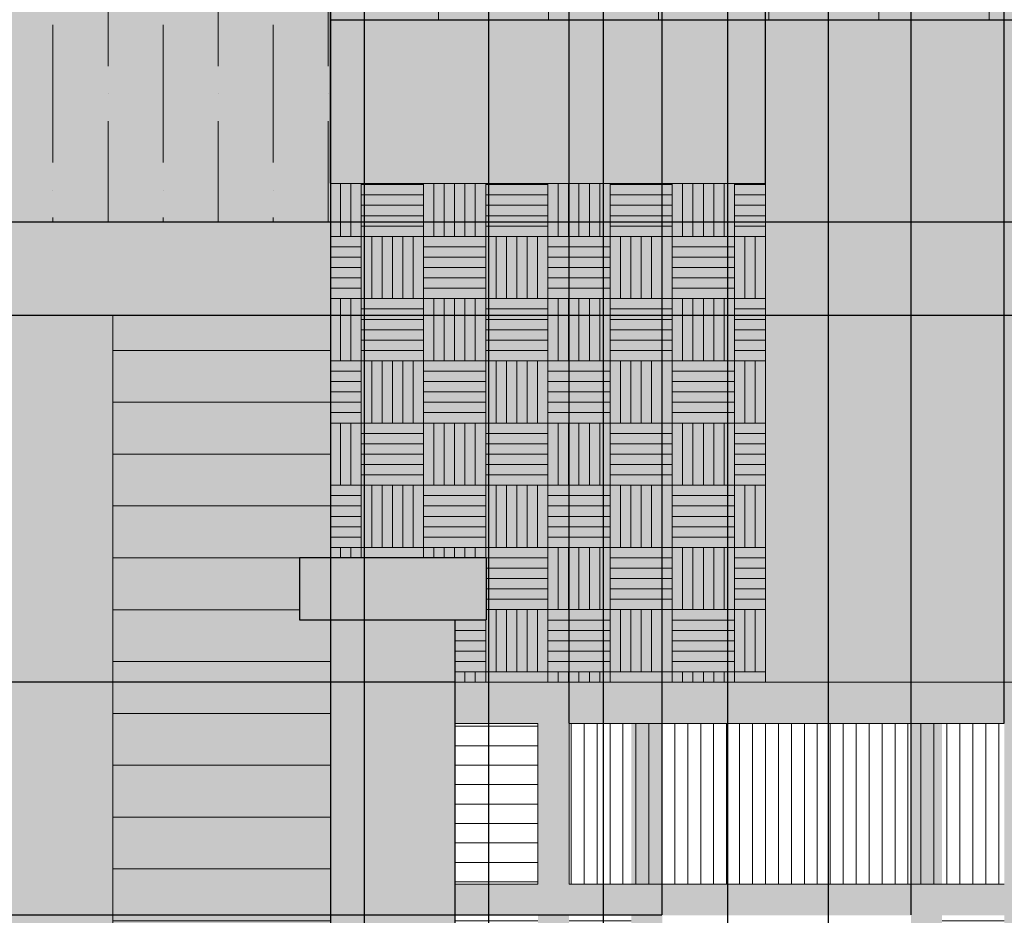
# Model space of a CAD drawing. Units: inches. Extents: x 180 to 1069, y 71 to 1267.
# Tile 3 of 8: x 546 to 736, y 301 to 474. Entities that reach past the tile are written whole.
import ezdxf

# ---------------------------------------------------------------- set-up
doc = ezdxf.new("R2010")
doc.units = ezdxf.units.IN
doc.header["$MEASUREMENT"] = 0
for name, color, linetype, lineweight in [('A-ANNO-DIMS', 2, 'Continuous', 18), ('A-COLS', 7, 'Continuous', 25), ('A-DOOR-GATE', 7, 'Continuous', 18), ('A-DOOR-PANL-PATT', 25, 'Continuous', 13), ('A-ELEV-FRAM', 7, 'Continuous', 25), ('A-WALL', 7, 'Continuous', 30), ('A-WALL-CLAD', 7, 'Continuous', 18), ('A-WALL-CLAD-JNTS-PATT', 18, 'Continuous', 13), ('A-WALL-CLAD-PATT', 26, 'Continuous', 13), ('A-WALL-PARQ-PATT', 69, 'Continuous', 13), ('A-WALL-SCRN-JNTS-PATT', 8, 'Continuous', 13)]:
    doc.layers.add(name, color=color, linetype=linetype, lineweight=lineweight)
for name, color, linetype, lineweight, true_color in [('A-DOOR-GATE-PATT', 18, 'Continuous', 13, 0x000000), ('A-DOOR-SHUT-PATT', 254, 'Continuous', 13, 0xb7d9eb), ('A-ELEV-BAND-PATT', 30, 'Continuous', 13, 0xf26722), ('A-ELEV-FRAM-PATT', 53, 'Continuous', 13, 0xefd648), ('A-ELEV-TRIM-PATT', 7, 'Continuous', 13, 0xffffff), ('A-WALL-RCSD-PATT', 251, 'Continuous', 13, 0x696959), ('A-WALL-SCRN-PATT', 251, 'Continuous', 13, 0x636466)]:
    doc.layers.add(name, color=color, linetype=linetype, lineweight=lineweight, true_color=true_color)
doc.styles.get("Standard").update_dxf_attribs({"font": 'arial.ttf'})
doc.dimstyles.get("Standard").update_dxf_attribs({"dimtxt": 6, "dimasz": 2, "dimexe": 0.18, "dimexo": 0.0625, "dimgap": 3, "dimtad": 0, "dimtih": 1, "dimtoh": 1, "dimdec": 0, "dimzin": 0, "dimdsep": 46, "dimlunit": 3, "dimtxsty": 'Standard', "dimcen": 0.09, "dimadec": 0, "dimazin": 0, "dimtfac": 1, "dimtdec": 0, "dimtofl": 0, "dimtmove": 0, "dimatfit": 3, "dimfxl": 1, "dimtolj": 1, "dimtzin": 0, "dimarcsym": 0})

# ---------------------------------------------------------------- blocks, each defined once
blk = doc.blocks.new('GATE-PIER-CAP')
for p, q in [((0, 12), (36, 12)), ((0, 12), (0, 0)), ((36, 12), (36, 0)), ((0, 0), (36, 0))]:
    blk.add_line(p, q)
blk = doc.blocks.new('*D31')
at = {"layer": 'A-ANNO-DIMS', "color": 0, "lineweight": -2, "transparency": 16777216}
for p, q in [((546.15, 416.82), (1056.28, 416.82)), ((1056.1, 414.82), (1056.1, 278.88)), ((1056.1, 130.82), (1056.1, 266.75)), ((546.15, 128.82), (1056.28, 128.82))]:
    blk.add_line(p, q, dxfattribs=at)
at = {"layer": 'A-ANNO-DIMS', "color": 0, "transparency": 16777216}
for points in [[(1055.77, 414.82), (1056.43, 414.82), (1056.1, 416.82)], [(1055.77, 130.82), (1056.43, 130.82), (1056.1, 128.82)]]:
    blk.add_solid(points, dxfattribs=at)
at = {"layer": 'Defpoints', "color": 0, "transparency": 16777216}
for p in [(546.09, 416.82), (1056.1, 416.82), (546.09, 128.82)]:
    blk.add_point(p, dxfattribs=at)
at = {"layer": 'A-ANNO-DIMS', "color": 0, "transparency": 16777216, "insert": (1056.1, 272.82), "char_height": 6, "attachment_point": 5}
blk.add_mtext('\\A1;288', dxfattribs=at)
blk = doc.blocks.new('*D32')
at = {"layer": 'A-ANNO-DIMS', "color": 0, "lineweight": -2, "transparency": 16777216}
for p, q in [((1056.1, 436.82), (1056.1, 438.82)), ((606.15, 434.82), (1056.28, 434.82)), ((546.15, 416.82), (1056.28, 416.82)), ((1056.1, 414.82), (1056.1, 412.82))]:
    blk.add_line(p, q, dxfattribs=at)
at = {"layer": 'A-ANNO-DIMS', "color": 0, "transparency": 16777216}
for points in [[(1055.77, 436.82), (1056.43, 436.82), (1056.1, 434.82)], [(1055.77, 414.82), (1056.43, 414.82), (1056.1, 416.82)]]:
    blk.add_solid(points, dxfattribs=at)
at = {"layer": 'Defpoints', "color": 0, "transparency": 16777216}
for p in [(606.09, 434.82), (1056.1, 434.82), (546.09, 416.82)]:
    blk.add_point(p, dxfattribs=at)
at = {"layer": 'A-ANNO-DIMS', "color": 0, "transparency": 16777216, "insert": (1056.1, 425.82), "char_height": 6, "attachment_point": 5}
blk.add_mtext('\\A1;18', dxfattribs=at)
blk = doc.blocks.new('*D39')
at = {"layer": 'A-ANNO-DIMS', "color": 0, "lineweight": -2, "transparency": 16777216}
for p, q in [((630.02, 346.05), (191.89, 346.05)), ((192.07, 344.05), (192.07, 249.5)), ((192.07, 142.82), (192.07, 237.37)), ((630.02, 140.82), (191.89, 140.82))]:
    blk.add_line(p, q, dxfattribs=at)
at = {"layer": 'A-ANNO-DIMS', "color": 0, "transparency": 16777216}
for points in [[(191.74, 344.05), (192.41, 344.05), (192.07, 346.05)], [(191.74, 142.82), (192.41, 142.82), (192.07, 140.82)]]:
    blk.add_solid(points, dxfattribs=at)
at = {"layer": 'Defpoints', "color": 0, "transparency": 16777216}
for p in [(192.07, 346.05), (630.09, 346.05), (630.09, 140.82)]:
    blk.add_point(p, dxfattribs=at)
at = {"layer": 'A-ANNO-DIMS', "color": 0, "transparency": 16777216, "insert": (192.07, 243.43), "char_height": 6, "attachment_point": 5}
blk.add_mtext('\\A1;205.23', dxfattribs=at)
blk = doc.blocks.new('*D40')
at = {"layer": 'A-ANNO-DIMS', "color": 0, "lineweight": -2, "transparency": 16777216}
for p, q in [((652.09, 338.11), (652.09, 1263.01)), ((654.09, 1262.83), (686.8, 1262.83)), ((734.09, 1262.83), (701.38, 1262.83)), ((736.09, 338.11), (736.09, 1263.01))]:
    blk.add_line(p, q, dxfattribs=at)
at = {"layer": 'A-ANNO-DIMS', "color": 0, "transparency": 16777216}
for points in [[(654.09, 1263.16), (654.09, 1262.5), (652.09, 1262.83)], [(734.09, 1263.16), (734.09, 1262.5), (736.09, 1262.83)]]:
    blk.add_solid(points, dxfattribs=at)
at = {"layer": 'Defpoints', "color": 0, "transparency": 16777216}
for p in [(736.09, 1262.83), (652.09, 338.05), (736.09, 338.05)]:
    blk.add_point(p, dxfattribs=at)
at = {"layer": 'A-ANNO-DIMS', "color": 0, "transparency": 16777216, "insert": (694.09, 1262.83), "char_height": 6, "attachment_point": 5}
blk.add_mtext('\\A1;84', dxfattribs=at)
blk = doc.blocks.new('*D42')
at = {"layer": 'A-ANNO-DIMS', "color": 0, "lineweight": -2, "transparency": 16777216}
for p, q in [((670.09, 301.11), (670.09, 1263.01)), ((672.09, 1262.83), (686.66, 1262.83)), ((716.09, 1262.83), (701.51, 1262.83)), ((718.09, 301.11), (718.09, 1263.01))]:
    blk.add_line(p, q, dxfattribs=at)
at = {"layer": 'A-ANNO-DIMS', "color": 0, "transparency": 16777216}
for points in [[(672.09, 1263.16), (672.09, 1262.5), (670.09, 1262.83)], [(716.09, 1263.16), (716.09, 1262.5), (718.09, 1262.83)]]:
    blk.add_solid(points, dxfattribs=at)
at = {"layer": 'Defpoints', "color": 0, "transparency": 16777216}
for p in [(718.09, 1262.83), (670.09, 301.05), (718.09, 301.05)]:
    blk.add_point(p, dxfattribs=at)
at = {"layer": 'A-ANNO-DIMS', "color": 0, "transparency": 16777216, "insert": (694.09, 1262.83), "char_height": 6, "attachment_point": 5}
blk.add_mtext('\\A1;48', dxfattribs=at)
blk = doc.blocks.new('*D43')
at = {"layer": 'A-ANNO-DIMS', "color": 0, "lineweight": -2, "transparency": 16777216}
for p, q in [((670.02, 301.05), (191.89, 301.05)), ((192.07, 299.05), (192.07, 295)), ((192.07, 278.82), (192.07, 282.87)), ((670.02, 276.82), (191.89, 276.82))]:
    blk.add_line(p, q, dxfattribs=at)
at = {"layer": 'A-ANNO-DIMS', "color": 0, "transparency": 16777216}
for points in [[(191.74, 299.05), (192.41, 299.05), (192.07, 301.05)], [(191.74, 278.82), (192.41, 278.82), (192.07, 276.82)]]:
    blk.add_solid(points, dxfattribs=at)
at = {"layer": 'Defpoints', "color": 0, "transparency": 16777216}
for p in [(670.09, 301.05), (192.07, 276.82), (670.09, 276.82)]:
    blk.add_point(p, dxfattribs=at)
at = {"layer": 'A-ANNO-DIMS', "color": 0, "transparency": 16777216, "insert": (192.07, 288.93), "char_height": 6, "attachment_point": 5}
blk.add_mtext('\\A1;24.23', dxfattribs=at)
blk = doc.blocks.new('*D44')
at = {"layer": 'A-ANNO-DIMS', "color": 0, "lineweight": -2, "transparency": 16777216}
for p, q in [((606.09, 442.3), (606.09, 1263.01)), ((608.09, 1262.83), (635.5, 1262.83)), ((688, 1262.83), (660.59, 1262.83)), ((690, 442.3), (690, 1263.01))]:
    blk.add_line(p, q, dxfattribs=at)
at = {"layer": 'A-ANNO-DIMS', "color": 0, "transparency": 16777216}
for points in [[(608.09, 1263.16), (608.09, 1262.5), (606.09, 1262.83)], [(688, 1263.16), (688, 1262.5), (690, 1262.83)]]:
    blk.add_solid(points, dxfattribs=at)
at = {"layer": 'Defpoints', "color": 0, "transparency": 16777216}
for p in [(690, 1262.83), (606.09, 442.24), (690, 442.24)]:
    blk.add_point(p, dxfattribs=at)
at = {"layer": 'A-ANNO-DIMS', "color": 0, "transparency": 16777216, "insert": (648.04, 1262.83), "char_height": 6, "attachment_point": 5}
blk.add_mtext('\\A1;83.91', dxfattribs=at)
blk = doc.blocks.new('*D45')
at = {"layer": 'A-ANNO-DIMS', "color": 0, "lineweight": -2, "transparency": 16777216}
for p, q in [((690, 442.3), (690, 1263.01)), ((692, 1262.83), (702.82, 1262.83)), ((739.89, 1262.83), (729.08, 1262.83)), ((741.89, 442.3), (741.89, 1263.01))]:
    blk.add_line(p, q, dxfattribs=at)
at = {"layer": 'A-ANNO-DIMS', "color": 0, "transparency": 16777216}
for points in [[(692, 1263.16), (692, 1262.5), (690, 1262.83)], [(739.89, 1263.16), (739.89, 1262.5), (741.89, 1262.83)]]:
    blk.add_solid(points, dxfattribs=at)
at = {"layer": 'Defpoints', "color": 0, "transparency": 16777216}
for p in [(741.89, 1262.83), (690, 442.24), (741.89, 442.24)]:
    blk.add_point(p, dxfattribs=at)
at = {"layer": 'A-ANNO-DIMS', "color": 0, "transparency": 16777216, "insert": (715.95, 1262.83), "char_height": 6, "attachment_point": 5}
blk.add_mtext('\\A1;51.89', dxfattribs=at)
blk = doc.blocks.new('*D58')
at = {"layer": 'A-ANNO-DIMS', "color": 0, "lineweight": -2, "transparency": 16777216}
for p, q in [((606.09, 1010.75), (606.09, 74.62)), ((498.09, 956.75), (498.09, 74.62)), ((500.09, 74.8), (542.74, 74.8)), ((604.09, 74.8), (561.44, 74.8))]:
    blk.add_line(p, q, dxfattribs=at)
at = {"layer": 'A-ANNO-DIMS', "color": 0, "transparency": 16777216}
for points in [[(500.09, 75.14), (500.09, 74.47), (498.09, 74.8)], [(604.09, 75.14), (604.09, 74.47), (606.09, 74.8)]]:
    blk.add_solid(points, dxfattribs=at)
at = {"layer": 'Defpoints', "color": 0, "transparency": 16777216}
for p in [(606.09, 1010.82), (498.09, 956.82), (606.09, 74.8)]:
    blk.add_point(p, dxfattribs=at)
at = {"layer": 'A-ANNO-DIMS', "color": 0, "transparency": 16777216, "insert": (552.09, 74.8), "char_height": 6, "attachment_point": 5}
blk.add_mtext('\\A1;108', dxfattribs=at)
blk = doc.blocks.new('*D59')
at = {"layer": 'A-ANNO-DIMS', "color": 0, "lineweight": -2, "transparency": 16777216}
for p, q in [((606.15, 1010.82), (1056.28, 1010.82)), ((1056.1, 1008.82), (1056.1, 728.88)), ((1056.1, 436.82), (1056.1, 716.75)), ((606.15, 434.82), (1056.28, 434.82))]:
    blk.add_line(p, q, dxfattribs=at)
at = {"layer": 'A-ANNO-DIMS', "color": 0, "transparency": 16777216}
for points in [[(1055.77, 1008.82), (1056.43, 1008.82), (1056.1, 1010.82)], [(1055.77, 436.82), (1056.43, 436.82), (1056.1, 434.82)]]:
    blk.add_solid(points, dxfattribs=at)
at = {"layer": 'Defpoints', "color": 0, "transparency": 16777216}
for p in [(606.09, 1010.82), (1056.1, 1010.82), (606.09, 434.82)]:
    blk.add_point(p, dxfattribs=at)
at = {"layer": 'A-ANNO-DIMS', "color": 0, "transparency": 16777216, "insert": (1056.1, 722.82), "char_height": 6, "attachment_point": 5}
blk.add_mtext('\\A1;576', dxfattribs=at)
blk = doc.blocks.new('*D60')
at = {"layer": 'A-ANNO-DIMS', "color": 0, "lineweight": -2, "transparency": 16777216}
for p, q in [((498.15, 488.82), (1056.28, 488.82)), ((1056.1, 486.82), (1056.1, 467.87)), ((1056.1, 436.82), (1056.1, 455.76)), ((606.15, 434.82), (1056.28, 434.82))]:
    blk.add_line(p, q, dxfattribs=at)
at = {"layer": 'A-ANNO-DIMS', "color": 0, "transparency": 16777216}
for points in [[(1055.77, 486.82), (1056.43, 486.82), (1056.1, 488.82)], [(1055.77, 436.82), (1056.43, 436.82), (1056.1, 434.82)]]:
    blk.add_solid(points, dxfattribs=at)
at = {"layer": 'Defpoints', "color": 0, "transparency": 16777216}
for p in [(498.09, 488.82), (606.09, 434.82), (1056.1, 434.82)]:
    blk.add_point(p, dxfattribs=at)
at = {"layer": 'A-ANNO-DIMS', "color": 0, "transparency": 16777216, "insert": (1056.1, 461.82), "char_height": 6, "attachment_point": 5}
blk.add_mtext('\\A1;54', dxfattribs=at)
blk = doc.blocks.new('*D65')
at = {"layer": 'A-ANNO-DIMS', "color": 0, "lineweight": -2, "transparency": 16777216}
for p, q in [((636.53, 557.75), (636.53, 74.62)), ((658.66, 557.75), (658.66, 74.62)), ((638.53, 74.8), (656.66, 74.8)), ((658.66, 74.8), (660.66, 74.8))]:
    blk.add_line(p, q, dxfattribs=at)
at = {"layer": 'A-ANNO-DIMS', "color": 0, "transparency": 16777216}
for points in [[(638.53, 75.14), (638.53, 74.47), (636.53, 74.8)], [(656.66, 75.14), (656.66, 74.47), (658.66, 74.8)]]:
    blk.add_solid(points, dxfattribs=at)
at = {"layer": 'Defpoints', "color": 0, "transparency": 16777216}
for p in [(636.53, 557.82), (658.66, 557.82), (658.66, 74.8)]:
    blk.add_point(p, dxfattribs=at)
at = {"layer": 'A-ANNO-DIMS', "color": 0, "transparency": 16777216, "insert": (676.17, 74.8), "char_height": 6, "attachment_point": 5}
blk.add_mtext('\\A1;22.133', dxfattribs=at)
blk = doc.blocks.new('*D66')
at = {"layer": 'A-ANNO-DIMS', "color": 0, "lineweight": -2, "transparency": 16777216}
for p, q in [((606.09, 647.75), (606.09, 74.62)), ((612.53, 557.75), (612.53, 74.62)), ((604.09, 74.8), (602.09, 74.8)), ((614.53, 74.8), (616.53, 74.8))]:
    blk.add_line(p, q, dxfattribs=at)
at = {"layer": 'A-ANNO-DIMS', "color": 0, "transparency": 16777216}
for points in [[(604.09, 75.14), (604.09, 74.47), (606.09, 74.8)], [(614.53, 75.14), (614.53, 74.47), (612.53, 74.8)]]:
    blk.add_solid(points, dxfattribs=at)
at = {"layer": 'Defpoints', "color": 0, "transparency": 16777216}
for p in [(606.09, 647.82), (612.53, 557.82), (612.53, 74.8)]:
    blk.add_point(p, dxfattribs=at)
at = {"layer": 'A-ANNO-DIMS', "color": 0, "transparency": 16777216, "insert": (627.32, 74.8), "char_height": 6, "attachment_point": 5}
blk.add_mtext('\\A1;6.44', dxfattribs=at)
blk = doc.blocks.new('*D67')
at = {"layer": 'A-ANNO-DIMS', "color": 0, "lineweight": -2, "transparency": 16777216}
for p, q in [((682.66, 557.75), (682.66, 74.62)), ((702.09, 557.75), (702.09, 74.62)), ((684.66, 74.8), (700.09, 74.8)), ((702.09, 74.8), (704.09, 74.8))]:
    blk.add_line(p, q, dxfattribs=at)
at = {"layer": 'A-ANNO-DIMS', "color": 0, "transparency": 16777216}
for points in [[(684.66, 75.14), (684.66, 74.47), (682.66, 74.8)], [(700.09, 75.14), (700.09, 74.47), (702.09, 74.8)]]:
    blk.add_solid(points, dxfattribs=at)
at = {"layer": 'Defpoints', "color": 0, "transparency": 16777216}
for p in [(682.66, 557.82), (702.09, 557.82), (702.09, 74.8)]:
    blk.add_point(p, dxfattribs=at)
at = {"layer": 'A-ANNO-DIMS', "color": 0, "transparency": 16777216, "insert": (719.26, 74.8), "char_height": 6, "attachment_point": 5}
blk.add_mtext('\\A1;19.427', dxfattribs=at)
blk = doc.blocks.new('*D68')
at = {"layer": 'A-ANNO-DIMS', "color": 0, "lineweight": -2, "transparency": 16777216}
for p, q in [((702.09, 557.75), (702.09, 74.62)), ((1002.09, 557.75), (1002.09, 74.62)), ((704.09, 74.8), (842.47, 74.8)), ((1000.09, 74.8), (861.7, 74.8))]:
    blk.add_line(p, q, dxfattribs=at)
at = {"layer": 'A-ANNO-DIMS', "color": 0, "transparency": 16777216}
for points in [[(704.09, 75.14), (704.09, 74.47), (702.09, 74.8)], [(1000.09, 75.14), (1000.09, 74.47), (1002.09, 74.8)]]:
    blk.add_solid(points, dxfattribs=at)
at = {"layer": 'Defpoints', "color": 0, "transparency": 16777216}
for p in [(702.09, 557.82), (1002.09, 557.82), (1002.09, 74.8)]:
    blk.add_point(p, dxfattribs=at)
at = {"layer": 'A-ANNO-DIMS', "color": 0, "transparency": 16777216, "insert": (852.09, 74.8), "char_height": 6, "attachment_point": 5}
blk.add_mtext('\\A1;300', dxfattribs=at)

msp = doc.modelspace()

# ---------------------------------------------------------------- hatches: boundary and pattern name
at = {"layer": 'A-DOOR-GATE-PATT'}
h = msp.add_hatch(color=256, dxfattribs=at)
h.dxf.hatch_style = 1
h.paths.add_polyline_path([(772.0875, 346.0477), (630.0875, 346.0477), (630.0875, 338.0477), (646.0875, 338.0477), (646.0875, 307.0477), (630.0875, 307.0477), (630.0875, 301.0477), (646.0875, 301.0477), (646.0875, 276.8159), (630.0875, 276.8159), (630.0875, 270.8159), (646.0875, 270.8159), (646.0875, 246.8159), (630.0875, 246.8159), (630.0875, 240.8159), (646.0875, 240.8159), (646.0875, 216.8159), (630.0875, 216.8159), (630.0875, 210.8159), (646.0875, 210.8159), (646.0875, 186.8159), (630.0875, 186.8159), (630.0875, 178.8159), (766.0875, 178.8159), (766.0875, 148.8159), (630.0875, 148.8159), (630.0875, 140.8159), (772.0875, 140.8159)])
h.paths.add_polyline_path([(670.0875, 338.0477), (718.0875, 338.0477), (718.0875, 307.0477), (670.0875, 307.0477)], flags=16)
h.paths.add_polyline_path([(664.0875, 338.0477), (664.0875, 307.0477), (652.0875, 307.0477), (652.0875, 338.0477)], flags=16)
h.paths.add_polyline_path([(670.0875, 301.0477), (718.0875, 301.0477), (718.0875, 276.8159), (670.0875, 276.8159)], flags=16)
h.paths.add_polyline_path([(664.0875, 301.0477), (664.0875, 276.8159), (652.0875, 276.8159), (652.0875, 301.0477)], flags=16)
h.paths.add_polyline_path([(724.0875, 338.0477), (736.0875, 338.0477), (736.0875, 307.0477), (724.0875, 307.0477)], flags=16)
h.paths.add_polyline_path([(724.0875, 301.0477), (736.0875, 301.0477), (736.0875, 276.8159), (724.0875, 276.8159)], flags=16)
h.paths.add_polyline_path([(670.0875, 270.8159), (718.0875, 270.8159), (718.0875, 246.8159), (670.0875, 246.8159)], flags=16)
h.paths.add_polyline_path([(664.0875, 270.8159), (664.0875, 246.8159), (652.0875, 246.8159), (652.0875, 270.8159)], flags=16)
h.paths.add_polyline_path([(742.0875, 338.0477), (766.0875, 338.0477), (766.0875, 307.0477), (742.0875, 307.0477)], flags=16)
h.paths.add_polyline_path([(742.0875, 301.0477), (766.0875, 301.0477), (766.0875, 276.8159), (742.0875, 276.8159)], flags=16)
h.paths.add_polyline_path([(724.0875, 270.8159), (736.0875, 270.8159), (736.0875, 246.8159), (724.0875, 246.8159)], flags=16)
h.paths.add_polyline_path([(670.0875, 240.8159), (718.0875, 240.8159), (718.0875, 216.8159), (670.0875, 216.8159)], flags=16)
h.paths.add_polyline_path([(664.0875, 240.8159), (664.0875, 216.8159), (652.0875, 216.8159), (652.0875, 240.8159)], flags=16)
h.paths.add_polyline_path([(742.0875, 270.8159), (766.0875, 270.8159), (766.0875, 246.8159), (742.0875, 246.8159)], flags=16)
h.paths.add_polyline_path([(724.0875, 240.8159), (736.0875, 240.8159), (736.0875, 216.8159), (724.0875, 216.8159)], flags=16)
h.paths.add_polyline_path([(742.0875, 240.8159), (766.0875, 240.8159), (766.0875, 216.8159), (742.0875, 216.8159)], flags=16)
h.paths.add_polyline_path([(670.0875, 210.8159), (718.0875, 210.8159), (718.0875, 186.8159), (670.0875, 186.8159)], flags=16)
h.paths.add_polyline_path([(664.0875, 210.8159), (664.0875, 186.8159), (652.0875, 186.8159), (652.0875, 210.8159)], flags=16)
h.paths.add_polyline_path([(724.0875, 210.8159), (736.0875, 210.8159), (736.0875, 186.8159), (724.0875, 186.8159)], flags=16)
h.paths.add_polyline_path([(742.0875, 210.8159), (766.0875, 210.8159), (766.0875, 186.8159), (742.0875, 186.8159)], flags=16)
h.paths.add_polyline_path([(918.0875, 346.0477), (776.0875, 346.0477), (776.0875, 140.8159), (918.0875, 140.8159), (918.0875, 148.8159), (782.0875, 148.8159), (782.0875, 178.8159), (918.0875, 178.8159), (918.0875, 186.8159), (902.0875, 186.8159), (902.0875, 210.8159), (918.0875, 210.8159), (918.0875, 216.8159), (902.0875, 216.8159), (902.0875, 240.8159), (918.0875, 240.8159), (918.0875, 246.8159), (902.0875, 246.8159), (902.0875, 270.8159), (918.0875, 270.8159), (918.0875, 276.8159), (902.0875, 276.8159), (902.0875, 301.0477), (918.0875, 301.0477), (918.0875, 307.0477), (902.0875, 307.0477), (902.0875, 338.0477), (918.0875, 338.0477)])
h.paths.add_polyline_path([(782.0875, 338.0477), (806.0875, 338.0477), (806.0875, 307.0477), (782.0875, 307.0477)], flags=16)
h.paths.add_polyline_path([(812.0875, 338.0477), (824.0875, 338.0477), (824.0875, 307.0477), (812.0875, 307.0477)], flags=16)
h.paths.add_polyline_path([(782.0875, 301.0477), (806.0875, 301.0477), (806.0875, 276.8159), (782.0875, 276.8159)], flags=16)
h.paths.add_polyline_path([(830.0875, 338.0477), (878.0875, 338.0477), (878.0875, 307.0477), (830.0875, 307.0477)], flags=16)
h.paths.add_polyline_path([(812.0875, 301.0477), (824.0875, 301.0477), (824.0875, 276.8159), (812.0875, 276.8159)], flags=16)
h.paths.add_polyline_path([(830.0875, 301.0477), (878.0875, 301.0477), (878.0875, 276.8159), (830.0875, 276.8159)], flags=16)
h.paths.add_polyline_path([(782.0875, 270.8159), (806.0875, 270.8159), (806.0875, 246.8159), (782.0875, 246.8159)], flags=16)
h.paths.add_polyline_path([(812.0875, 270.8159), (824.0875, 270.8159), (824.0875, 246.8159), (812.0875, 246.8159)], flags=16)
h.paths.add_polyline_path([(830.0875, 270.8159), (878.0875, 270.8159), (878.0875, 246.8159), (830.0875, 246.8159)], flags=16)
h.paths.add_polyline_path([(782.0875, 240.8159), (806.0875, 240.8159), (806.0875, 216.8159), (782.0875, 216.8159)], flags=16)
h.paths.add_polyline_path([(884.0875, 338.0477), (896.0875, 338.0477), (896.0875, 307.0477), (884.0875, 307.0477)], flags=16)
h.paths.add_polyline_path([(812.0875, 240.8159), (824.0875, 240.8159), (824.0875, 216.8159), (812.0875, 216.8159)], flags=16)
h.paths.add_polyline_path([(884.0875, 301.0477), (896.0875, 301.0477), (896.0875, 276.8159), (884.0875, 276.8159)], flags=16)
h.paths.add_polyline_path([(830.0875, 240.8159), (878.0875, 240.8159), (878.0875, 216.8159), (830.0875, 216.8159)], flags=16)
h.paths.add_polyline_path([(884.0875, 270.8159), (896.0875, 270.8159), (896.0875, 246.8159), (884.0875, 246.8159)], flags=16)
h.paths.add_polyline_path([(782.0875, 210.8159), (806.0875, 210.8159), (806.0875, 186.8159), (782.0875, 186.8159)], flags=16)
h.paths.add_polyline_path([(812.0875, 210.8159), (824.0875, 210.8159), (824.0875, 186.8159), (812.0875, 186.8159)], flags=16)
h.paths.add_polyline_path([(830.0875, 210.8159), (878.0875, 210.8159), (878.0875, 186.8159), (830.0875, 186.8159)], flags=16)
h.paths.add_polyline_path([(884.0875, 240.8159), (896.0875, 240.8159), (896.0875, 216.8159), (884.0875, 216.8159)], flags=16)
h.paths.add_polyline_path([(884.0875, 210.8159), (896.0875, 210.8159), (896.0875, 186.8159), (884.0875, 186.8159)], flags=16)
h = msp.add_hatch(dxfattribs=at)
h.set_pattern_fill('ANSI31', color=256, scale=30, angle=135)
h.paths.add_polyline_path([(646.0875, 338.0477), (630.0875, 338.0477), (630.0875, 307.0477), (646.0875, 307.0477)])
h.paths.add_polyline_path([(646.0875, 301.0477), (630.0875, 301.0477), (630.0875, 276.8159), (646.0875, 276.8159)])
h.paths.add_polyline_path([(664.0875, 301.0477), (652.0875, 301.0477), (652.0875, 276.8159), (664.0875, 276.8159)])
h.paths.add_polyline_path([(664.0875, 270.8159), (652.0875, 270.8159), (652.0875, 246.8159), (664.0875, 246.8159)])
h.paths.add_polyline_path([(646.0875, 270.8159), (630.0875, 270.8159), (630.0875, 246.8159), (646.0875, 246.8159)])
h.paths.add_polyline_path([(646.0875, 240.8159), (630.0875, 240.8159), (630.0875, 216.8159), (646.0875, 216.8159)])
h.paths.add_polyline_path([(664.0875, 240.8159), (652.0875, 240.8159), (652.0875, 216.8159), (664.0875, 216.8159)])
h.paths.add_polyline_path([(664.0875, 210.8159), (652.0875, 210.8159), (652.0875, 186.8159), (664.0875, 186.8159)])
h.paths.add_polyline_path([(646.0875, 210.8159), (630.0875, 210.8159), (630.0875, 186.8159), (646.0875, 186.8159)])
h.paths.add_polyline_path([(736.0875, 301.0477), (724.0875, 301.0477), (724.0875, 276.8159), (736.0875, 276.8159)])
h.paths.add_polyline_path([(766.0875, 301.0477), (742.0875, 301.0477), (742.0875, 276.8159), (766.0875, 276.8159)])
h.paths.add_polyline_path([(766.0875, 270.8159), (742.0875, 270.8159), (742.0875, 246.8159), (766.0875, 246.8159)])
h.paths.add_polyline_path([(766.0875, 338.0477), (742.0875, 338.0477), (742.0875, 307.0477), (766.0875, 307.0477)])
h.paths.add_polyline_path([(736.0875, 270.8159), (724.0875, 270.8159), (724.0875, 246.8159), (736.0875, 246.8159)])
h.paths.add_polyline_path([(736.0875, 240.8159), (724.0875, 240.8159), (724.0875, 216.8159), (736.0875, 216.8159)])
h.paths.add_polyline_path([(766.0875, 240.8159), (742.0875, 240.8159), (742.0875, 216.8159), (766.0875, 216.8159)])
h.paths.add_polyline_path([(766.0875, 210.8159), (742.0875, 210.8159), (742.0875, 186.8159), (766.0875, 186.8159)])
h.paths.add_polyline_path([(736.0875, 210.8159), (724.0875, 210.8159), (724.0875, 186.8159), (736.0875, 186.8159)])
h.paths.add_polyline_path([(806.0875, 210.8159), (782.0875, 210.8159), (782.0875, 186.8159), (806.0875, 186.8159)])
h.paths.add_polyline_path([(806.0875, 240.8159), (782.0875, 240.8159), (782.0875, 216.8159), (806.0875, 216.8159)])
h.paths.add_polyline_path([(806.0875, 270.8159), (782.0875, 270.8159), (782.0875, 246.8159), (806.0875, 246.8159)])
h.paths.add_polyline_path([(806.0875, 301.0477), (782.0875, 301.0477), (782.0875, 276.8159), (806.0875, 276.8159)])
h.paths.add_polyline_path([(806.0875, 338.0477), (782.0875, 338.0477), (782.0875, 307.0477), (806.0875, 307.0477)])
h.paths.add_polyline_path([(824.0875, 301.0477), (812.0875, 301.0477), (812.0875, 276.8159), (824.0875, 276.8159)])
h.paths.add_polyline_path([(824.0875, 270.8159), (812.0875, 270.8159), (812.0875, 246.8159), (824.0875, 246.8159)])
h.paths.add_polyline_path([(824.0875, 240.8159), (812.0875, 240.8159), (812.0875, 216.8159), (824.0875, 216.8159)])
h.paths.add_polyline_path([(824.0875, 210.8159), (812.0875, 210.8159), (812.0875, 186.8159), (824.0875, 186.8159)])
h.paths.add_polyline_path([(918.0875, 338.0477), (902.0875, 338.0477), (902.0875, 307.0477), (918.0875, 307.0477)])
h.paths.add_polyline_path([(918.0875, 301.0477), (902.0875, 301.0477), (902.0875, 276.8159), (918.0875, 276.8159)])
h.paths.add_polyline_path([(918.0875, 270.8159), (902.0875, 270.8159), (902.0875, 246.8159), (918.0875, 246.8159)])
h.paths.add_polyline_path([(918.0875, 240.8159), (902.0875, 240.8159), (902.0875, 216.8159), (918.0875, 216.8159)])
h.paths.add_polyline_path([(918.0875, 210.8159), (902.0875, 210.8159), (902.0875, 186.8159), (918.0875, 186.8159)])
h.paths.add_polyline_path([(896.0875, 210.8159), (884.0875, 210.8159), (884.0875, 186.8159), (896.0875, 186.8159)])
h.paths.add_polyline_path([(896.0875, 240.8159), (884.0875, 240.8159), (884.0875, 216.8159), (896.0875, 216.8159)])
h.paths.add_polyline_path([(896.0875, 270.8159), (884.0875, 270.8159), (884.0875, 246.8159), (896.0875, 246.8159)])
h.paths.add_polyline_path([(896.0875, 301.0477), (884.0875, 301.0477), (884.0875, 276.8159), (896.0875, 276.8159)])
h = msp.add_hatch(dxfattribs=at)
h.set_pattern_fill('ANSI31', color=256, scale=20, angle=45)
h.paths.add_polyline_path([(736.0875, 338.0477), (724.0875, 338.0477), (664.0875, 338.0477), (652.0875, 338.0477), (652.0875, 307.0477), (664.0875, 307.0477), (724.0875, 307.0477), (736.0875, 307.0477)])
h.paths.add_polyline_path([(896.0875, 338.0477), (884.0875, 338.0477), (824.0875, 338.0477), (812.0875, 338.0477), (812.0875, 307.0477), (830.0875, 307.0477), (884.0875, 307.0477), (896.0875, 307.0477)])
at = {"layer": 'A-DOOR-PANL-PATT'}
h = msp.add_hatch(color=256, dxfattribs=at)
h.dxf.hatch_style = 1
h.paths.add_polyline_path([(690.001, 442.2382), (606.0875, 442.2382), (606.0875, 416.8159), (606.0875, 370.0477), (636.0875, 370.0477), (636.0875, 358.0477), (630.0875, 358.0477), (630.0875, 346.0477), (690.001, 346.0477)])
at = {"layer": 'A-DOOR-SHUT-PATT'}
h = msp.add_hatch(color=256, dxfattribs=at)
h.dxf.hatch_style = 1
h.paths.add_polyline_path([(546.0875, 416.8159), (306.0875, 416.8159), (306.0875, 140.8159), (546.0875, 140.8159)])
h.paths.add_polyline_path([(306.0875, 416.8159), (288.0875, 416.8159), (288.0875, 128.8159), (306.0875, 128.8159)])
h.paths.add_polyline_path([(546.0875, 140.8159), (306.0875, 140.8159), (306.0875, 128.8159), (546.0875, 128.8159)])
h.paths.add_polyline_path([(564.0875, 416.8159), (546.0875, 416.8159), (546.0875, 140.8159), (546.0875, 128.8159), (564.0875, 128.8159)])
at = {"layer": 'A-ELEV-BAND-PATT'}
h = msp.add_hatch(color=256, dxfattribs=at)
h.dxf.hatch_style = 1
h.paths.add_polyline_path([(1002.0875, 1148.8159), (726.0875, 1148.8159), (726.0875, 1130.8159), (954.0875, 1130.8159), (954.0875, 947.2513), (978.0875, 947.2513), (978.0875, 1130.8159), (1002.0875, 1130.8159)])
h.paths.add_polyline_path([(654.0875, 1148.8159), (354.0875, 1148.8159), (354.0875, 1130.8159), (654.0875, 1130.8159)])
h.paths.add_polyline_path([(606.0875, 434.8159), (246.0875, 434.8159), (246.0875, 416.8159), (606.0875, 416.8159)])
h.paths.add_polyline_path([(978.0875, 845.8159), (726.0875, 845.8159), (726.0875, 791.8159), (978.0875, 791.8159)])
at = {"layer": 'A-ELEV-FRAM-PATT'}
h = msp.add_hatch(color=256, dxfattribs=at)
h.dxf.hatch_style = 1
h.paths.add_polyline_path([(354.0875, 1184.8159), (654.0875, 1184.8159), (654.0875, 974.8159), (726.0875, 974.8159), (726.0875, 1208.8159), (288.0875, 1208.8159), (288.0875, 897.6348), (304.7188, 897.6348), (304.7188, 883.4805), (288.0875, 883.4805), (288.0875, 866.8025), (304.7188, 866.8025), (304.7188, 852.6482), (288.0875, 852.6482), (288.0875, 835.9702), (304.7188, 835.9702), (304.7188, 821.8159), (288.0875, 821.8159), (288.0875, 805.1379), (304.7188, 805.1379), (304.7188, 790.9836), (288.0875, 790.9836), (288.0875, 774.3056), (304.7188, 774.3056), (304.7188, 760.1513), (288.0875, 760.1513), (288.0875, 743.4733), (304.7188, 743.4733), (304.7188, 729.319), (288.0875, 729.319), (288.0875, 434.8159), (354.0875, 434.8159), (354.0875, 456.1177), (317.1892, 456.1177), (317.1892, 516.1177), (354.0875, 516.1177), (354.0875, 924.0304), (317.1892, 924.0304), (317.1892, 984.0304), (354.0875, 984.0304)])
h.paths.add_polyline_path([(1002.0875, 869.8159), (702.0875, 869.8159), (702.0875, 791.8159), (726.0875, 791.8159), (726.0875, 845.8159), (978.0875, 845.8159), (978.0875, 581.8159), (726.0875, 581.8159), (726.0875, 647.8159), (702.0875, 647.8159), (702.0875, 557.8159), (1002.0875, 557.8159)])
h.paths.add_polyline_path([(906.0875, 1080.2003), (882.0875, 1080.2003), (882.0875, 1056.2003), (906.0875, 1056.2003)])
h.paths.add_polyline_path([(906.0875, 996.2003), (882.0875, 996.2003), (882.0875, 972.2003), (906.0875, 972.2003)])
h.paths.add_polyline_path([(636.5273, 869.8159), (612.5273, 869.8159), (612.5273, 845.8159), (636.5273, 845.8159)], flags=17)
h.paths.add_polyline_path([(682.6602, 869.8159), (658.6602, 869.8159), (658.6602, 845.8159), (682.6602, 845.8159)], flags=17)
h.paths.add_polyline_path([(636.5273, 581.8159), (612.5273, 581.8159), (612.5273, 557.8159), (636.5273, 557.8159)], flags=17)
h.paths.add_polyline_path([(682.6602, 581.8159), (658.6602, 581.8159), (658.6602, 557.8159), (682.6602, 557.8159)], flags=17)
h.paths.add_polyline_path([(942.0875, 358.0477), (918.0875, 358.0477), (918.0875, 128.8159), (942.0875, 128.8159)])
h.paths.add_polyline_path([(630.0875, 358.0477), (606.0875, 358.0477), (606.0875, 128.8159), (630.0875, 128.8159)])
at = {"layer": 'A-ELEV-TRIM-PATT'}
h = msp.add_hatch(color=256, dxfattribs=at)
h.dxf.hatch_style = 1
h.paths.add_polyline_path([(467.1892, 516.1177), (317.1892, 516.1177), (317.1892, 456.1177), (467.1892, 456.1177)])
h.paths.add_polyline_path([(458.1892, 507.1177), (458.1892, 465.1177), (326.1892, 465.1177), (326.1892, 507.1177)], flags=16)
h.paths.add_polyline_path([(354.0875, 816.0741), (354.0875, 804.0741), (426.0875, 804.0741), (426.0875, 636.0741), (354.0875, 636.0741), (354.0875, 624.0741), (438.0875, 624.0741), (438.0875, 816.0741)])
h.paths.add_polyline_path([(317.1892, 924.0304), (467.1892, 924.0304), (467.1892, 984.0304), (317.1892, 984.0304)])
h.paths.add_polyline_path([(326.1892, 933.0304), (326.1892, 975.0304), (458.1892, 975.0304), (458.1892, 933.0304)], flags=16)
h.paths.add_polyline_path([(304.7188, 897.6348), (262.2193, 897.6348), (262.2193, 883.4805), (304.7188, 883.4805)])
h.paths.add_polyline_path([(304.7188, 866.8025), (262.2193, 866.8025), (262.2193, 852.6482), (304.7188, 852.6482)])
h.paths.add_polyline_path([(304.7188, 835.9702), (262.2193, 835.9702), (262.2193, 821.8159), (304.7188, 821.8159)])
h.paths.add_polyline_path([(304.7188, 805.1379), (262.2193, 805.1379), (262.2193, 790.9836), (304.7188, 790.9836)])
h.paths.add_polyline_path([(304.7188, 774.3056), (262.2193, 774.3056), (262.2193, 760.1513), (304.7188, 760.1513)])
h.paths.add_polyline_path([(304.7188, 743.4733), (262.2193, 743.4733), (262.2193, 729.319), (304.7188, 729.319)])
h.paths.add_polyline_path([(600.0875, 370.0477), (600.0875, 358.0477), (636.0875, 358.0477), (636.0875, 370.0477)])
h.paths.add_polyline_path([(912.0875, 370.0477), (912.0875, 358.0477), (948.0875, 358.0477), (948.0875, 370.0477)])
at = {"layer": 'A-WALL-CLAD-JNTS-PATT'}
h = msp.add_hatch(dxfattribs=at)
h.set_pattern_fill('ANSI31', color=256, scale=80, angle=135)
h.paths.add_polyline_path([(288.0875, 416.8159), (246.0875, 416.8159), (246.0875, 128.8159), (288.0875, 128.8159)])
h.paths.add_polyline_path([(606.0875, 358.0477), (600.0875, 358.0477), (600.0875, 370.0477), (606.0875, 370.0477), (606.0875, 416.8159), (564.0875, 416.8159), (564.0875, 128.8159), (606.0875, 128.8159)])
h.paths.add_polyline_path([(288.0875, 729.319), (262.2193, 729.319), (262.2193, 743.4733), (288.0875, 743.4733), (288.0875, 760.1513), (262.2193, 760.1513), (262.2193, 774.3056), (288.0875, 774.3056), (288.0875, 790.9836), (262.2193, 790.9836), (262.2193, 805.1379), (288.0875, 805.1379), (288.0875, 821.8159), (262.2193, 821.8159), (262.2193, 835.9702), (288.0875, 835.9702), (288.0875, 852.6482), (262.2193, 852.6482), (262.2193, 866.8025), (288.0875, 866.8025), (288.0875, 883.4805), (262.2193, 883.4805), (262.2193, 897.6348), (288.0875, 897.6348), (288.0875, 1208.8159), (246.0875, 1208.8159), (246.0875, 434.8159), (288.0875, 434.8159)])
at = {"layer": 'A-WALL-CLAD-PATT'}
h = msp.add_hatch(color=256, dxfattribs=at)
h.dxf.hatch_style = 1
h.paths.add_polyline_path([(606.0875, 358.0477), (600.0875, 358.0477), (600.0875, 370.0477), (606.0875, 370.0477), (606.0875, 416.8159), (564.0875, 416.8159), (564.0875, 128.8159), (606.0875, 128.8159)])
at = {"layer": 'A-WALL-PARQ-PATT'}
h = msp.add_hatch(dxfattribs=at)
h.set_pattern_fill('AR-PARQ1', color=256, angle=270)
h.paths.add_polyline_path([(690.001, 442.2382), (606.0875, 442.2382), (606.0875, 416.8159), (606.0875, 370.0477), (636.0875, 370.0477), (636.0875, 358.0477), (630.0875, 358.0477), (630.0875, 346.0477), (690.001, 346.0477)])
at = {"layer": 'A-WALL-RCSD-PATT'}
h = msp.add_hatch(color=256, dxfattribs=at)
h.dxf.hatch_style = 1
h.paths.add_polyline_path([(741.8928, 442.2382), (825.8928, 442.2382), (825.8928, 364.2866), (894.0875, 473.8159), (606.0875, 473.8159), (606.0875, 442.2382), (690.001, 442.2382), (690.001, 346.0477), (741.8928, 346.0477)])
at = {"layer": 'A-WALL-SCRN-JNTS-PATT'}
h = msp.add_hatch(dxfattribs=at)
h.set_pattern_fill('ANSI36', color=256, scale=85, angle=45)
h.paths.add_polyline_path([(606.0875, 938.8159), (798.0875, 938.8159), (798.0875, 869.8159), (834.0875, 869.8159), (834.0875, 974.8159), (606.0875, 974.8159), (606.0875, 1010.8159), (354.0875, 1010.8159), (354.0875, 984.0304), (467.1892, 984.0304), (467.1892, 956.8159), (498.0875, 956.8159), (498.0875, 488.8159), (467.1892, 488.8159), (467.1892, 456.1177), (354.0875, 456.1177), (354.0875, 434.8159), (606.0875, 434.8159), (606.0875, 473.8159), (834.0875, 473.8159), (834.0875, 557.8159), (798.0875, 557.8159), (798.0875, 509.8159), (606.0875, 509.8159)])
at = {"layer": 'A-WALL-SCRN-PATT'}
h = msp.add_hatch(color=256, dxfattribs=at)
h.dxf.hatch_style = 1
h.paths.add_polyline_path([(606.0875, 938.8159), (798.0875, 938.8159), (798.0875, 869.8159), (834.0875, 869.8159), (834.0875, 974.8159), (606.0875, 974.8159), (606.0875, 1010.8159), (354.0875, 1010.8159), (354.0875, 984.0304), (467.1892, 984.0304), (467.1892, 956.8159), (498.0875, 956.8159), (498.0875, 488.8159), (467.1892, 488.8159), (467.1892, 456.1177), (354.0875, 456.1177), (354.0875, 434.8159), (606.0875, 434.8159), (606.0875, 473.8159), (834.0875, 473.8159), (834.0875, 557.8159), (798.0875, 557.8159), (798.0875, 509.8159), (606.0875, 509.8159)])
h.paths.add_polyline_path([(367.1892, 507.1177), (326.1892, 507.1177), (326.1892, 465.1177), (367.1892, 465.1177)])
h.paths.add_polyline_path([(411.1892, 507.1177), (373.1892, 507.1177), (373.1892, 465.1177), (411.1892, 465.1177)], flags=17)
h.paths.add_polyline_path([(458.1892, 507.1177), (417.1892, 507.1177), (417.1892, 465.1177), (458.1892, 465.1177)], flags=17)
h.paths.add_polyline_path([(426.0875, 672.0741), (354.0875, 672.0741), (354.0875, 636.0741), (426.0875, 636.0741)], flags=17)
h.paths.add_polyline_path([(426.0875, 760.0741), (354.0875, 760.0741), (354.0875, 680.0741), (426.0875, 680.0741)], flags=17)
h.paths.add_polyline_path([(426.0875, 804.0741), (354.0875, 804.0741), (354.0875, 768.0741), (426.0875, 768.0741)], flags=17)
h.paths.add_polyline_path([(367.1892, 975.0304), (326.1892, 975.0304), (326.1892, 933.0304), (367.1892, 933.0304)])
h.paths.add_polyline_path([(411.1892, 975.0304), (373.1892, 975.0304), (373.1892, 933.0304), (411.1892, 933.0304)], flags=17)
h.paths.add_polyline_path([(458.1892, 975.0304), (417.1892, 975.0304), (417.1892, 933.0304), (458.1892, 933.0304)], flags=17)

# ---------------------------------------------------------------- linework, layer by layer
at = {"layer": 'A-COLS'}
for p, q in [((606.0875, 358.0477), (606.0875, 128.8159)), ((630.0875, 358.0477), (630.0875, 128.8159))]:
    msp.add_line(p, q, dxfattribs=at)
at = {"layer": 'A-DOOR-GATE'}
for p, q in [((630.0875, 346.0477), (776.0875, 346.0477)), ((630.0875, 338.0477), (646.0875, 338.0477)), ((646.0875, 338.0477), (646.0875, 307.0477)), ((652.0875, 338.0477), (652.0875, 307.0477)), ((652.0875, 338.0477), (664.0875, 338.0477)), ((664.0875, 338.0477), (724.0875, 338.0477)), ((724.0875, 338.0477), (736.0875, 338.0477)), ((630.0875, 307.0477), (646.0875, 307.0477)), ((652.0875, 307.0477), (664.0875, 307.0477)), ((664.0875, 307.0477), (724.0875, 307.0477)), ((724.0875, 307.0477), (736.0875, 307.0477))]:
    msp.add_line(p, q, dxfattribs=at)
at = {"layer": 'A-ELEV-FRAM'}
for p, q in [((246.0875, 434.8159), (606.0875, 434.8159)), ((246.0875, 416.8159), (606.0875, 416.8159))]:
    msp.add_line(p, q, dxfattribs=at)
at = {"layer": 'A-WALL'}
msp.add_line((606.0875, 473.8159), (978.0875, 473.8159), dxfattribs=at)
at = {"layer": 'A-WALL-CLAD'}
for p, q in [((606.0875, 416.8159), (606.0875, 473.8159)), ((606.0875, 442.2382), (690.001, 442.2382)), ((690.001, 442.2382), (690.001, 346.0477)), ((564.0875, 416.8159), (564.0875, 128.8159)), ((606.0875, 416.8159), (606.0875, 370.0477))]:
    msp.add_line(p, q, dxfattribs=at)

# ---------------------------------------------------------------- block references
at = {"layer": 'A-COLS'}
msp.add_blockref('GATE-PIER-CAP', (600.0875, 358.0477), dxfattribs=at)

# ---------------------------------------------------------------- dimensions: what is measured, and where the dimension line sits
at = {"layer": 'A-ANNO-DIMS'}
for base, p1, p2, override, picture, middle in [((690.001, 1262.8294), (606.0875, 442.2382), (690.001, 442.2382), {"dimdec": 2, "dimlfac": 1, "dimrnd": 0, "dimzin": 0, "dimdsep": 46, "dimlunit": 2}, '*D44', (648.0442, 1262.8294)), ((736.0875, 1262.8294), (652.0875, 338.0477), (736.0875, 338.0477), {"dimdec": 0, "dimlfac": 1, "dimrnd": 0, "dimzin": 0, "dimdsep": 46, "dimlunit": 2}, '*D40', (694.0875, 1262.8294)), ((718.0875, 1262.8294), (670.0875, 301.0477), (718.0875, 301.0477), {"dimdec": 0, "dimlfac": 1, "dimrnd": 0, "dimzin": 0, "dimdsep": 46, "dimlunit": 2}, '*D42', (694.0875, 1262.8294)), ((741.8928, 1262.8294), (690.001, 442.2382), (741.8928, 442.2382), {"dimdec": 2, "dimlfac": 1, "dimrnd": 0, "dimzin": 0, "dimdsep": 46, "dimlunit": 2}, '*D45', (715.9469, 1262.8294)), ((606.0875, 74.8024), (498.0875, 956.8159), (606.0875, 1010.8159), {"dimdec": 0, "dimlfac": 1, "dimrnd": 0, "dimzin": 0, "dimdsep": 46, "dimlunit": 2}, '*D58', (552.0875, 74.8024)), ((612.5273, 74.8024), (606.0875, 647.8159), (612.5273, 557.8159), {"dimdec": 2, "dimlfac": 1, "dimrnd": 0, "dimzin": 0, "dimdsep": 46, "dimlunit": 2}, '*D66', (627.324, 74.8024)), ((658.6602, 74.8024), (636.5273, 557.8159), (658.6602, 557.8159), {"dimdec": 3, "dimlfac": 1, "dimrnd": 0, "dimzin": 0, "dimdsep": 46, "dimlunit": 2}, '*D65', (676.1657, 74.8024)), ((702.0875, 74.8024), (682.6602, 557.8159), (702.0875, 557.8159), {"dimdec": 3, "dimlfac": 1, "dimrnd": 0, "dimzin": 0, "dimdsep": 46, "dimlunit": 2}, '*D67', (719.2594, 74.8024)), ((1002.0875, 74.8024), (702.0875, 557.8159), (1002.0875, 557.8159), {"dimdec": 0, "dimlfac": 1, "dimrnd": 0, "dimzin": 0, "dimdsep": 46, "dimlunit": 2}, '*D68', (852.0875, 74.8024))]:
    dim = msp.add_linear_dim(base=base, p1=p1, p2=p2, dimstyle='Standard', override=override, dxfattribs=at)
    dim.commit()
    dim.dimension.update_dxf_attribs({"geometry": picture, "text_midpoint": middle})
for base, p1, p2, override, picture, middle in [((1056.101, 1010.8159), (606.0875, 434.8159), (606.0875, 1010.8159), {"dimdec": 0, "dimlfac": 1, "dimrnd": 0, "dimzin": 0, "dimdsep": 46, "dimlunit": 2}, '*D59', (1056.101, 722.8159)), ((1056.101, 434.8159), (498.0875, 488.8159), (606.0875, 434.8159), {"dimdec": 0, "dimlfac": 1, "dimrnd": 0, "dimzin": 0, "dimdsep": 46, "dimlunit": 2}, '*D60', (1056.101, 461.8159)), ((1056.101, 434.8159), (546.0875, 416.8159), (606.0875, 434.8159), {"dimdec": 0, "dimlfac": 1, "dimrnd": 0, "dimzin": 0, "dimdsep": 46, "dimlunit": 2}, '*D32', (1056.101, 425.8159)), ((1056.101, 416.8159), (546.0875, 128.8159), (546.0875, 416.8159), {"dimdec": 0, "dimlfac": 1, "dimrnd": 0, "dimzin": 0, "dimdsep": 46, "dimlunit": 2}, '*D31', (1056.101, 272.8159)), ((192.074, 346.0477), (630.0875, 140.8159), (630.0875, 346.0477), {"dimdec": 2, "dimlfac": 1, "dimrnd": 0, "dimzin": 0, "dimdsep": 46, "dimlunit": 2}, '*D39', (192.074, 243.4318)), ((192.074, 276.8159), (670.0875, 301.0477), (670.0875, 276.8159), {"dimdec": 2, "dimlfac": 1, "dimrnd": 0, "dimzin": 0, "dimdsep": 46, "dimlunit": 2}, '*D43', (192.074, 288.9318))]:
    dim = msp.add_linear_dim(base=base, p1=p1, p2=p2, angle=90, dimstyle='Standard', override=override, dxfattribs=at)
    dim.commit()
    dim.dimension.update_dxf_attribs({"geometry": picture, "text_midpoint": middle})

doc.saveas('drawing.dxf')
